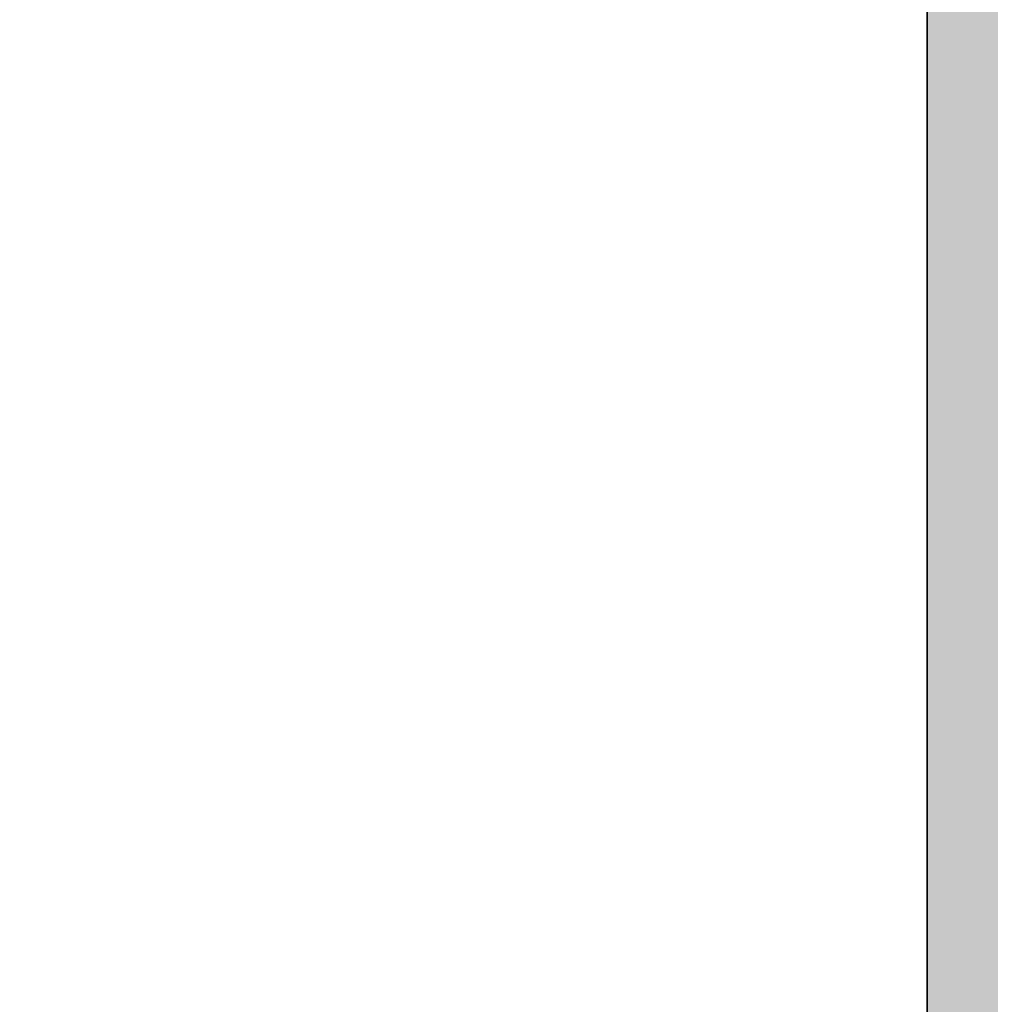
# Model space of a CAD drawing. Units: inches. Extents: x 2696 to 3240, y 1564 to 2310.
# Tile 4 of 76: x 2874.74 to 2893.42, y 1633.53 to 1652.49. Entities that reach past the tile are written whole.
import ezdxf

# ---------------------------------------------------------------- set-up
doc = ezdxf.new("R2010")
doc.units = ezdxf.units.IN
for name, color, linetype, lineweight in [('A-ANNO-DIMS', 3, 'Continuous', 18), ('A-WALL', 7, 'Continuous', 35), ('A-WALL-PATT', 9, 'Continuous', 13)]:
    doc.layers.add(name, color=color, linetype=linetype, lineweight=lineweight)
doc.styles.add('TIMES NEW', font='times.ttf')
doc.dimstyles.new('Siddhuu', dxfattribs={"dimtxt": 6, "dimasz": 2.5, "dimexe": 1.25, "dimexo": 0.625, "dimtad": 1, "dimdec": 1, "dimlunit": 4, "dimtxsty": 'TIMES NEW', "dimcen": 2.5, "dimclrd": 256, "dimclre": 1, "dimclrt": 7, "dimadec": 0, "dimazin": 0, "dimtfac": 1, "dimtdec": 1, "dimtmove": 0, "dimatfit": 3, "dimfxl": 1, "dimtolj": 1, "dimlwd": -1, "dimarcsym": 0})

# ---------------------------------------------------------------- blocks, each defined once
blk = doc.blocks.new('*D57')
at = {"layer": 'A-ANNO-DIMS', "color": 1, "lineweight": -2, "transparency": 16777216}
for p, q in [((2754.611, 2018.576), (2754.611, 1568.951)), ((2956.709, 2018.576), (2956.709, 1568.951))]:
    blk.add_line(p, q, dxfattribs=at)
at = {"layer": 'A-ANNO-DIMS', "transparency": 16777216}
blk.add_line((2757.111, 1570.201), (2954.209, 1570.201), dxfattribs=at)
for points in [[(2757.111, 1570.618), (2757.111, 1569.784), (2754.611, 1570.201)], [(2954.209, 1570.618), (2954.209, 1569.784), (2956.709, 1570.201)]]:
    blk.add_solid(points, dxfattribs=at)
at = {"layer": 'Defpoints', "color": 0, "transparency": 16777216}
for p in [(2754.611, 2019.201), (2956.709, 2019.201), (2956.709, 1570.201)]:
    blk.add_point(p, dxfattribs=at)
at = {"layer": 'A-ANNO-DIMS', "color": 7, "transparency": 16777216, "insert": (2855.66, 1573.878), "char_height": 6, "attachment_point": 5, "style": 'TIMES NEW'}
blk.add_mtext('\\A1;16\'-10"', dxfattribs=at)
blk = doc.blocks.new('*D69')
at = {"layer": 'A-ANNO-DIMS', "color": 1, "lineweight": -2, "transparency": 16777216}
for p, q in [((2841.889, 2261.576), (2841.889, 1568.951)), ((2905.91, 2261.576), (2905.91, 1568.951))]:
    blk.add_line(p, q, dxfattribs=at)
at = {"layer": 'A-ANNO-DIMS', "transparency": 16777216}
blk.add_line((2844.389, 1570.201), (2903.41, 1570.201), dxfattribs=at)
for points in [[(2844.389, 1570.618), (2844.389, 1569.784), (2841.889, 1570.201)], [(2903.41, 1570.618), (2903.41, 1569.784), (2905.91, 1570.201)]]:
    blk.add_solid(points, dxfattribs=at)
at = {"layer": 'Defpoints', "color": 0, "transparency": 16777216}
for p in [(2841.889, 2262.201), (2905.91, 2262.201), (2905.91, 1570.201)]:
    blk.add_point(p, dxfattribs=at)
at = {"layer": 'A-ANNO-DIMS', "color": 7, "transparency": 16777216, "insert": (2873.9, 1573.878), "char_height": 6, "attachment_point": 5, "style": 'TIMES NEW'}
blk.add_mtext('\\A1;5\'-4"', dxfattribs=at)

msp = doc.modelspace()

# ---------------------------------------------------------------- hatches: boundary and pattern name
at = {"layer": 'A-WALL-PATT', "transparency": 33554556}
h = msp.add_hatch(color=256, dxfattribs=at)
h.dxf.hatch_style = 1
h.paths.add_polyline_path([(2879.111, 2253.201), (2905.91, 2253.201), (2905.91, 2262.201), (2841.889, 2262.201), (2841.889, 2253.201), (2870.111, 2253.201), (2870.111, 2176.601), (2965.709, 2176.601), (2965.709, 2206.701), (2973.583, 2206.701), (2973.583, 2215.701), (2965.709, 2215.701), (2965.709, 2262.201), (2929.91, 2262.201), (2929.91, 2253.201), (2956.709, 2253.201), (2956.709, 2185.601), (2879.111, 2185.601)])
h.paths.add_polyline_path([(2782.834, 2262.201), (2745.611, 2262.201), (2745.611, 2228.729), (2754.611, 2228.729), (2754.611, 2253.201), (2782.834, 2253.201)])
h.paths.add_polyline_path([(2754.611, 2136.201), (2965.709, 2136.201), (2965.709, 2145.201), (2879.111, 2145.201), (2879.111, 2147.074), (2877.34, 2147.074), (2870.111, 2147.074), (2870.111, 2145.201), (2754.611, 2145.201), (2754.611, 2169.674), (2745.611, 2169.674), (2745.611, 2000.201), (2754.611, 2000.201), (2754.611, 2019.201), (2849.083, 2019.201), (2849.083, 2023.701), (2841.209, 2023.701), (2841.209, 2051.827), (2836.709, 2051.827), (2836.709, 2023.701), (2754.611, 2023.701), (2754.611, 2091.201), (2836.709, 2091.201), (2836.709, 2087.827), (2841.209, 2087.827), (2841.209, 2095.701), (2754.611, 2095.701)])
h.paths.add_polyline_path([(2965.709, 2136.201), (2956.709, 2136.201), (2956.709, 2023.701), (2885.083, 2023.701), (2885.083, 2019.201), (2956.709, 2019.201), (2956.709, 1950.575), (2965.709, 1950.575), (2965.709, 1980.201), (2973.583, 1980.201), (2973.583, 1989.201), (2965.709, 1989.201)])
h.paths.add_polyline_path([(2754.611, 1906.701), (2880.209, 1906.701), (2884.709, 1906.701), (2956.709, 1906.701), (2956.709, 1792.701), (2944.709, 1792.701), (2944.709, 1783.701), (2956.709, 1783.701), (2956.709, 1740.201), (2884.709, 1740.201), (2884.709, 1783.701), (2896.709, 1783.701), (2896.709, 1792.701), (2884.709, 1792.701), (2884.709, 1846.701), (2880.209, 1846.701), (2880.209, 1740.201), (2754.611, 1740.201), (2754.611, 1777.201), (2745.611, 1777.201), (2745.611, 1692.701), (2754.611, 1692.701), (2754.611, 1731.201), (2956.709, 1731.201), (2956.709, 1723.327), (2965.709, 1723.327), (2965.709, 1884.201), (2973.583, 1884.201), (2973.583, 1893.201), (2965.709, 1893.201), (2965.709, 1914.575), (2956.709, 1914.575), (2956.709, 1911.201), (2754.611, 1911.201), (2754.611, 1930.201), (2745.611, 1930.201), (2745.611, 1817.201), (2754.611, 1817.201), (2754.611, 1854.201), (2826.611, 1854.201), (2826.611, 1868.827), (2822.111, 1868.827), (2822.111, 1858.701), (2754.611, 1858.701)])
h.paths.add_polyline_path([(2965.709, 1656.201), (3008.237, 1656.201), (3008.237, 1665.201), (2965.709, 1665.201), (2965.709, 1693.327), (2956.709, 1693.327), (2956.709, 1686.201), (2934.583, 1686.201), (2934.583, 1681.701), (2956.709, 1681.701), (2956.709, 1614.201), (2896.709, 1614.201), (2896.709, 1681.701), (2904.583, 1681.701), (2904.583, 1686.201), (2892.209, 1686.201), (2892.209, 1614.201), (2858.41, 1614.201), (2858.41, 1605.201), (2965.709, 1605.201)])
h.paths.add_polyline_path([(2788.41, 1614.201), (2754.611, 1614.201), (2754.611, 1652.701), (2745.611, 1652.701), (2745.611, 1605.201), (2788.41, 1605.201)])
h.paths.add_polyline_path([(3199.611, 1633.048), (3190.611, 1633.048), (3190.611, 1614.201), (3082.611, 1614.201), (3082.611, 1665.201), (3070.237, 1665.201), (3070.237, 1656.201), (3078.111, 1656.201), (3078.111, 1605.201), (3199.611, 1605.201)])
h.paths.add_polyline_path([(3199.611, 1702.048), (3190.611, 1702.048), (3190.611, 1699.701), (3106.611, 1699.701), (3106.611, 1747.701), (3190.611, 1747.701), (3190.611, 1752.201), (3082.611, 1752.201), (3082.611, 1760.075), (3078.111, 1760.075), (3078.111, 1747.701), (3102.111, 1747.701), (3102.111, 1699.701), (3078.111, 1699.701), (3078.111, 1695.201), (3190.611, 1695.201), (3190.611, 1676.355), (3199.611, 1676.355)])
h.paths.add_polyline_path([(3199.611, 1783.201), (3190.611, 1783.201), (3190.611, 1745.355), (3199.611, 1745.355)])
h.paths.add_polyline_path([(3082.611, 1884.201), (3190.611, 1884.201), (3190.611, 1853.201), (3199.611, 1853.201), (3199.611, 1901.701), (3190.611, 1901.701), (3190.611, 1893.201), (3005.583, 1893.201), (3005.583, 1891.281), (3005.583, 1884.201), (3078.111, 1884.201), (3078.111, 1792.075), (3082.611, 1792.075)])
h.paths.add_polyline_path([(3199.611, 1994.701), (3190.611, 1994.701), (3190.611, 1989.201), (3073.709, 1989.201), (3073.709, 2034.201), (3069.209, 2034.201), (3069.209, 1989.201), (3005.583, 1989.201), (3005.583, 1980.201), (3190.611, 1980.201), (3190.611, 1971.701), (3199.611, 1971.701)])
h.paths.add_polyline_path([(3199.611, 2155.201), (3190.611, 2155.201), (3190.611, 2064.701), (3199.611, 2064.701)])
h.paths.add_polyline_path([(3190.611, 2074.701), (3106.611, 2074.701), (3106.611, 2122.701), (3190.611, 2122.701), (3190.611, 2127.201), (3082.709, 2127.201), (3082.709, 2135.075), (3073.709, 2135.075), (3073.709, 2122.701), (3102.111, 2122.701), (3102.111, 2074.701), (3069.209, 2074.701), (3069.209, 2070.201), (3190.611, 2070.201)])
h.paths.add_polyline_path([(3082.709, 2253.201), (3190.611, 2253.201), (3190.611, 2225.201), (3199.611, 2225.201), (3199.611, 2262.201), (3073.709, 2262.201), (3073.709, 2215.701), (3035.583, 2215.701), (3035.583, 2206.701), (3073.709, 2206.701), (3073.709, 2171.075), (3082.709, 2171.075)])

# ---------------------------------------------------------------- linework, layer by layer
at = {"layer": 'A-WALL'}
msp.add_line((2892.209, 1686.201), (2892.209, 1614.201), dxfattribs=at)

# ---------------------------------------------------------------- dimensions: what is measured, and where the dimension line sits
at = {"layer": 'A-ANNO-DIMS'}
for base, p1, p2, picture, middle in [((2905.91, 1570.201), (2841.889, 2262.201), (2905.91, 2262.201), '*D69', (2873.9, 1573.878)), ((2956.709, 1570.201), (2754.611, 2019.201), (2956.709, 2019.201), '*D57', (2855.66, 1573.878))]:
    dim = msp.add_linear_dim(base=base, p1=p1, p2=p2, dimstyle='Siddhuu', override={"dimdec": 1, "dimlfac": 1, "dimrnd": 0, "dimzin": 1, "dimdsep": 46, "dimlunit": 4, "dimfrac": 2}, dxfattribs=at)
    dim.commit()
    dim.dimension.update_dxf_attribs({"geometry": picture, "text_midpoint": middle})

doc.saveas('drawing.dxf')
